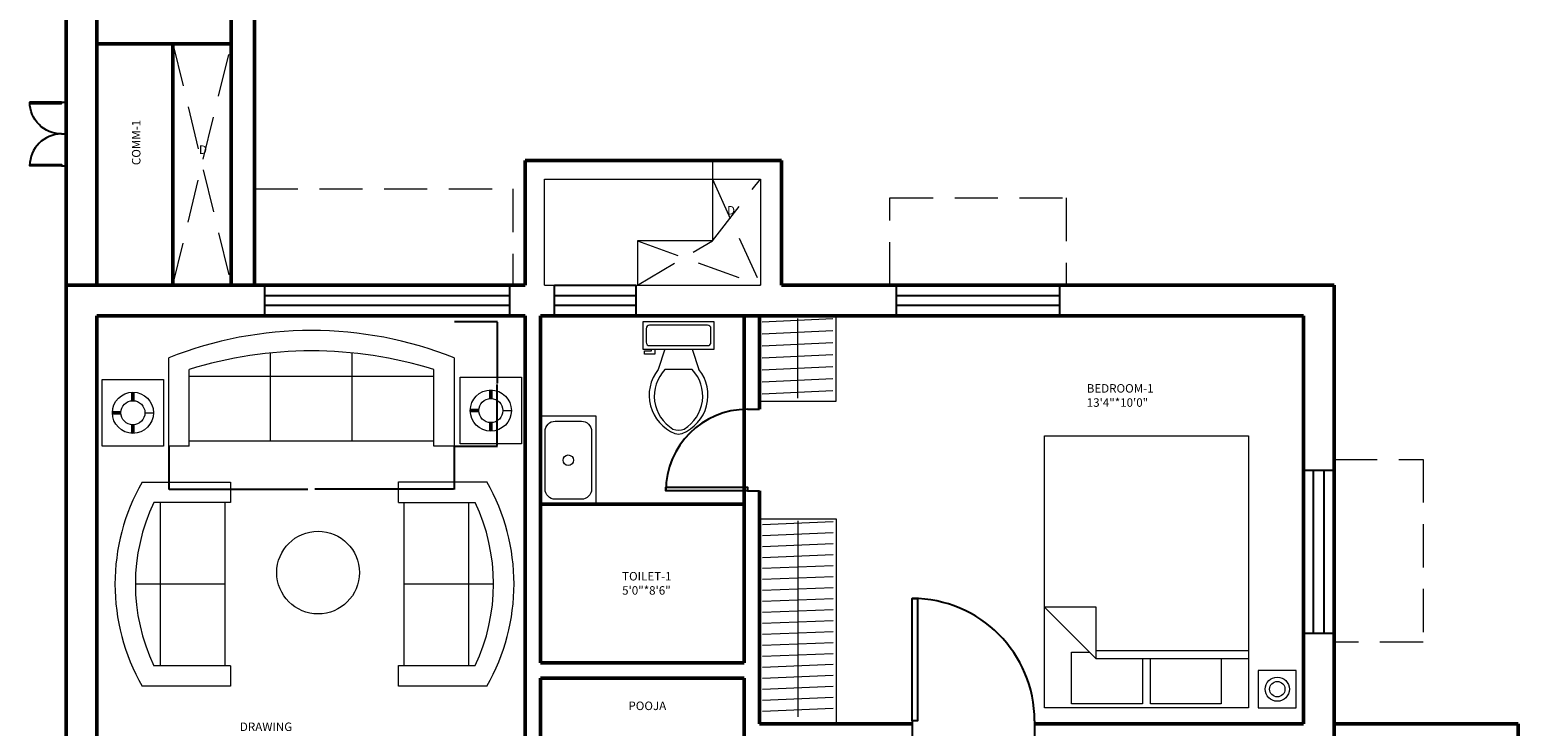
# Model space of a CAD drawing. Units: inches. Extents: x 4795 to 6024, y 2716 to 5025.
# Tile 8 of 19: x 5517 to 5955, y 3611 to 3816. Entities that reach past the tile are written whole.
import ezdxf

# ---------------------------------------------------------------- set-up
doc = ezdxf.new("R2010")
doc.units = ezdxf.units.IN
doc.linetypes.add('DASHED', pattern=[19.05, 12.7, -6.35])
for name, color, linetype, lineweight in [('A-ANNO-DIMS', 2, 'Continuous', 18), ('A-ANNO-TEXT', 7, 'Continuous', 18), ('A-AREA-IDEN', 3, 'Continuous', 18), ('A-DOOR', 4, 'Continuous', 25), ('A-FLOR-FIXT', 9, 'Continuous', 18), ('A-FURN', 8, 'Continuous', 18), ('A-GLAZ', 4, 'Continuous', 25), ('A-WALL', 7, 'Continuous', 50), ('A-WALL-OVHD', 8, 'DASHED', 18)]:
    doc.layers.add(name, color=color, linetype=linetype, lineweight=lineweight)
doc.styles.get("Standard").update_dxf_attribs({"font": 'arial.ttf'})
doc.dimstyles.get("Standard").update_dxf_attribs({"dimtxt": 0.18, "dimasz": 0.18, "dimexe": 0.18, "dimexo": 0.0625, "dimgap": 0.09, "dimtad": 0, "dimtih": 1, "dimtoh": 1, "dimdec": 4, "dimzin": 0, "dimdsep": 46, "dimtxsty": 'Standard', "dimcen": 0.09, "dimadec": 0, "dimazin": 0, "dimtfac": 1, "dimtdec": 4, "dimtofl": 0, "dimtmove": 0, "dimatfit": 3, "dimfxl": 1, "dimtolj": 1, "dimtzin": 0, "dimarcsym": 0})

# ---------------------------------------------------------------- blocks, each defined once
blk = doc.blocks.new('*U2')
for p, q in [((0, 0), (0, -6)), ((40, 0), (40, -6))]:
    blk.add_line(p, q)
blk.add_lwpolyline([(0, 0), (0, 40), (1.75, 40), (1.75, 0)], close=True)
blk.add_arc((0, 0), 40, 0, 90)
blk = doc.blocks.new('Sofa - Roundback 7 ft.')
for p, q in [((-12.00002, -32.4421), (-12.00003, -6.5971)), ((11.99997, -32.4421), (11.99998, -6.5971)), ((-36.000027, -34), (-36.000027, -11.4696)), ((35.99998, -34), (35.99998, -11.4696)), ((-35.999844, -13.3819), (35.9998, -13.3819)), ((-36.000027, -32.4421), (35.99998, -32.4421))]:
    blk.add_line(p, q)
for points in [[(-36.000027, -34), (-42.000027, -34), (-42.000027, -8)], [(41.99998, -8), (41.99998, -34), (35.99998, -34)]]:
    blk.add_lwpolyline(points)
for centre, radius, start, end in [((0, -114.25), 114.25, 68.43141, 111.5686), ((-0.00001, -127.1968), 121.1968, 72.72033, 107.2797)]:
    blk.add_arc(centre, radius, start, end)
blk = doc.blocks.new('Sofa - Roundback Loveseat 5 ft.')
for p, q in [((0, -32.44198), (0, -5.99998)), ((-24, -33.99998), (-24, -11.46958)), ((24.00004, -33.99998), (24.00004, -11.46958)), ((-23.9998, -13.38178), (23.99986, -13.38178)), ((-24, -32.44198), (24.00004, -32.44198))]:
    blk.add_line(p, q)
for points in [[(-24, -33.99998), (-30, -33.99998), (-30, -7.99998)], [(30.00004, -7.99998), (30.00004, -33.99998), (24.00004, -33.99998)]]:
    blk.add_lwpolyline(points)
for centre, radius, start, end in [((0, -60.24998), 60.24998, 60.13715, 119.8628), ((0, -61.38438), 55.38444, 64.32083, 115.6792)]:
    blk.add_arc(centre, radius, start, end)
blk = doc.blocks.new('Toilet - top')
for p, q in [((9.5, -6), (9.5, -2)), ((-10, -8.5), (-8, -8.5)), ((-10, -9.5), (-10, -8.5)), ((-8, -8.5), (-8, -8)), ((-7, -8), (-7, -9.5)), ((-4, -8), (-6, -14)), ((4, -8), (6, -14)), ((-7, -9.5), (-10, -9.5)), ((4, -14), (-4, -14))]:
    blk.add_line(p, q)
blk.add_lwpolyline([(10.5, -8), (10.5, 0), (-10.5, 0), (-10.5, -8)], close=True)
for points in [[(-9.5, -2), (-9.5, -6)], [(8.5, -1), (-8.5, -1)], [(-8.5, -7), (8.5, -7)]]:
    blk.add_lwpolyline(points)
for centre, radius, start, end in [((-8.62, -1.88), 0.884, 81.8699, 188.1301), ((8.62, -1.88), 0.884, 351.8699, 98.1301), ((-8.62, -6.12), 0.884, 171.8699, 278.1301), ((8.62, -6.12), 0.884, 261.8699, 8.1301), ((3.52, -21.58), 12.17, 141.4691, 247.9714), ((4.2, -21.82), 11.33, 136.3677, 238.9468), ((-3.52, -21.58), 12.17, 292.0284, 38.5307), ((-4.2, -21.82), 11.33, 301.053, 43.6321), ((0, -27.88), 4, 245.7318, 294.2682), ((0, -29), 4, 254.8605, 285.1395)]:
    blk.add_arc(centre, radius, start, end)
blk = doc.blocks.new('Bed - Queen')
for p, q in [((0, -80.00003), (0, 0)), ((0, 0), (59.99999, 0)), ((59.99999, 0), (59.99999, -80.00003)), ((7.99999, -1.2), (28.79998, -1.2)), ((7.99999, -14.4), (7.99999, -1.2)), ((28.79998, -1.2), (28.79998, -14.4)), ((31.19999, -1.2), (51.99999, -1.2)), ((31.19999, -14.4), (31.19999, -1.2)), ((51.99999, -1.2), (51.99999, -16.4)), ((0, -14.4), (44.8, -14.4)), ((44.8, -16.8), (0, -16.8)), ((59.99999, -29.6), (44.8, -14.4)), ((44.8, -14.4), (44.8, -29.6)), ((51.99999, -16.4), (46.79936, -16.4)), ((44.8, -29.6), (59.99999, -29.6)), ((59.99999, -80.00003), (0, -80.00003))]:
    blk.add_line(p, q)
blk = doc.blocks.new('WIN-48')
for p, q in [((0, 0), (0, 48)), ((0, 48), (9, 48)), ((3, 0), (3, 48)), ((6, 48), (6, 0)), ((9, 48), (9, 0)), ((9, 0), (0, 0))]:
    blk.add_line(p, q)
blk = doc.blocks.new('WIN-72')
for p, q in [((0, 0), (0, 9)), ((0, 9), (72, 9)), ((72, 9), (72, 0)), ((0, 6), (72, 6)), ((72, 3), (0, 3)), ((72, 0), (0, 0))]:
    blk.add_line(p, q)
blk = doc.blocks.new('WIN-24')
for p, q in [((0, 0), (0, 9)), ((0, 9), (24, 9)), ((24, 9), (24, 0)), ((0, 6), (24, 6)), ((24, 3), (0, 3)), ((24, 0), (0, 0))]:
    blk.add_line(p, q)
blk = doc.blocks.new('*D41')
at = {"layer": 'A-ANNO-DIMS', "color": 0, "lineweight": -2, "transparency": 16777216}
for p, q in [((5558.35, 3693.06), (5558.35, 3680.34)), ((5642.35, 3693.06), (5642.35, 3680.34)), ((5558.53, 3680.52), (5599.32, 3680.52)), ((5642.17, 3680.52), (5601.38, 3680.52))]:
    blk.add_line(p, q, dxfattribs=at)
at = {"layer": 'A-ANNO-DIMS', "color": 0, "lineweight": 100, "transparency": 16777216}
for points in [[(5558.53, 3680.55), (5558.53, 3680.49), (5558.35, 3680.52)], [(5642.17, 3680.55), (5642.17, 3680.49), (5642.35, 3680.52)]]:
    blk.add_solid(points, dxfattribs=at)
at = {"layer": 'DEFPOINTS', "color": 0, "lineweight": 100, "transparency": 16777216}
for p in [(5558.35, 3693.12), (5642.35, 3693.12), (5642.35, 3680.52)]:
    blk.add_point(p, dxfattribs=at)
at = {"layer": 'A-ANNO-DIMS', "color": 0, "transparency": 16777216, "insert": (5600.35, 3680.52), "char_height": 0.18, "attachment_point": 5}
blk.add_mtext("\\A1;SOFA 7' 84 TYP.", dxfattribs=at)
blk = doc.blocks.new('*D42')
at = {"layer": 'A-ANNO-DIMS', "color": 0, "lineweight": -2, "transparency": 16777216}
for p, q in [((5642.41, 3729.79), (5655.13, 3729.79)), ((5654.95, 3729.61), (5654.95, 3711.64)), ((5654.95, 3693.3), (5654.95, 3711.28)), ((5642.41, 3693.12), (5655.13, 3693.12))]:
    blk.add_line(p, q, dxfattribs=at)
at = {"layer": 'A-ANNO-DIMS', "color": 0, "lineweight": 100, "transparency": 16777216}
for points in [[(5654.92, 3729.61), (5654.98, 3729.61), (5654.95, 3729.79)], [(5654.92, 3693.3), (5654.98, 3693.3), (5654.95, 3693.12)]]:
    blk.add_solid(points, dxfattribs=at)
at = {"layer": 'DEFPOINTS', "color": 0, "lineweight": 100, "transparency": 16777216}
for p in [(5642.35, 3729.79), (5654.95, 3729.79), (5642.35, 3693.12)]:
    blk.add_point(p, dxfattribs=at)
at = {"layer": 'A-ANNO-DIMS', "color": 0, "transparency": 16777216, "insert": (5654.95, 3711.46), "char_height": 0.18, "attachment_point": 5}
blk.add_mtext('\\A1;37 TYP.', dxfattribs=at)

msp = doc.modelspace()

# ---------------------------------------------------------------- linework, layer by layer
at = {"layer": 'A-FLOR-FIXT'}
msp.add_lwpolyline([(5667.72, 3676.04), (5684.08, 3676.04), (5684.08, 3701.96), (5667.72, 3701.96)], close=True, dxfattribs=at)
msp.add_lwpolyline([(5672.08, 3700.46), (5679.77, 3700.46, -0.414214), (5682.77, 3697.46), (5682.77, 3680.5, -0.414214), (5679.77, 3677.5), (5672.08, 3677.5, -0.414214), (5669.08, 3680.5), (5669.08, 3697.46, -0.414214)], format="xyb", close=True, dxfattribs=at)
msp.add_circle((5675.92, 3688.98), 1.55, dxfattribs=at)
at = {"layer": 'A-FURN'}
for p, q in [((5718.34, 3777.12), (5718.34, 3771.66)), ((5668.93, 3740.43), (5668.93, 3771.66)), ((5668.93, 3771.66), (5732.5, 3771.66)), ((5718.34, 3771.66), (5718.34, 3753.53)), ((5732.5, 3771.66), (5732.5, 3740.43)), ((5718.34, 3753.53), (5696.25, 3753.53)), ((5696.25, 3753.53), (5696.25, 3740.43)), ((5668.93, 3740.43), (5732.5, 3740.43)), ((5754.73, 3706.3), (5754.73, 3731.43)), ((5732.94, 3729.68), (5753.73, 3730.61)), ((5732.94, 3726.15), (5753.73, 3727.08)), ((5743.33, 3730.69), (5743.33, 3707.22)), ((5732.94, 3722.62), (5753.73, 3723.55)), ((5732.94, 3719.1), (5753.73, 3720.03)), ((5732.94, 3715.57), (5753.73, 3716.5)), ((5732.94, 3712.05), (5753.73, 3712.98)), ((5732.22, 3706.3), (5754.73, 3706.3)), ((5732.94, 3708.52), (5753.73, 3709.45)), ((5551.36, 3702.94), (5553.87, 3702.94)), ((5656.67, 3703.58), (5659.18, 3703.58)), ((5732.22, 3671.71), (5754.73, 3671.71)), ((5733.04, 3670.11), (5753.82, 3670.93)), ((5743.43, 3671.14), (5743.43, 3613.55)), ((5754.73, 3671.71), (5754.73, 3611.43)), ((5733.04, 3666.88), (5753.82, 3667.7)), ((5733.04, 3663.66), (5753.82, 3664.48)), ((5733.04, 3660.43), (5753.82, 3661.25)), ((5733.04, 3657.2), (5753.82, 3658.02)), ((5733.04, 3653.97), (5753.82, 3654.79)), ((5733.04, 3650.74), (5753.82, 3651.56)), ((5733.04, 3647.52), (5753.82, 3648.34)), ((5733.04, 3644.29), (5753.82, 3645.11)), ((5733.04, 3641.06), (5753.82, 3641.88)), ((5733.04, 3637.83), (5753.82, 3638.65)), ((5733.04, 3634.6), (5753.82, 3635.42)), ((5733.04, 3631.38), (5753.82, 3632.2)), ((5733.04, 3628.15), (5753.82, 3628.97)), ((5733.04, 3624.92), (5753.82, 3625.74)), ((5733.04, 3621.69), (5753.82, 3622.51)), ((5733.04, 3618.46), (5753.82, 3619.28)), ((5733.04, 3615.24), (5753.82, 3616.06))]:
    msp.add_line(p, q, dxfattribs=at)
for points in [[(5556.84, 3693.12), (5538.81, 3693.12), (5538.81, 3712.75), (5556.84, 3712.75)], [(5662.14, 3693.77), (5644.11, 3693.77), (5644.11, 3713.4), (5662.14, 3713.4)], [(5878.95, 3616.19), (5890.13, 3616.19), (5890.13, 3627.14), (5878.95, 3627.14)]]:
    msp.add_lwpolyline(points, close=True, dxfattribs=at)
for centre, radius in [((5653.13, 3703.58), 6.05), ((5547.82, 3702.94), 6.05), ((5547.82, 3702.94), 3.54), ((5653.13, 3703.58), 3.54), ((5602.31, 3655.94), 12.16), ((5884.54, 3621.66), 3.55), ((5884.54, 3621.66), 2.26)]:
    msp.add_circle(centre, radius, dxfattribs=at)
at = {"layer": 'A-WALL'}
for p, q in [((5537.22, 3929.81), (5537.22, 3740.43)), ((5528.22, 3920.81), (5528.22, 3351.93)), ((5576.74, 3920.81), (5576.74, 3740.43)), ((5583.63, 3920.81), (5583.63, 3740.43)), ((5537.22, 3811.38), (5576.74, 3811.38)), ((5559.58, 3811.38), (5559.58, 3740.43)), ((5663.22, 3740.43), (5663.22, 3777.12)), ((5663.22, 3777.12), (5732.22, 3777.12)), ((5732.22, 3777.12), (5738.7, 3777.12)), ((5738.7, 3777.12), (5738.7, 3740.43)), ((5528.22, 3740.43), (5663.22, 3740.43)), ((5738.7, 3740.43), (5901.22, 3740.43)), ((5901.22, 3740.43), (5901.22, 3606.93)), ((5537.22, 3731.43), (5663.22, 3731.43)), ((5537.22, 3731.43), (5537.22, 3551.43)), ((5663.22, 3731.43), (5663.22, 3606.93)), ((5667.72, 3731.43), (5667.72, 3629.43)), ((5667.72, 3731.43), (5892.22, 3731.43)), ((5727.72, 3731.43), (5727.72, 3629.43)), ((5732.22, 3731.43), (5732.22, 3703.97)), ((5892.22, 3731.43), (5892.22, 3611.43)), ((5653.13, 3709.64), (5653.13, 3707.12)), ((5547.82, 3708.99), (5547.82, 3706.48)), ((5541.77, 3702.94), (5544.28, 3702.94)), ((5647.07, 3703.58), (5649.59, 3703.58)), ((5547.82, 3699.4), (5547.82, 3696.88)), ((5653.13, 3700.04), (5653.13, 3697.53)), ((5732.22, 3679.97), (5732.22, 3611.43)), ((5667.72, 3676.04), (5727.72, 3676.04)), ((5667.72, 3629.43), (5727.72, 3629.43)), ((5667.72, 3624.93), (5727.72, 3624.93)), ((5667.72, 3624.93), (5667.72, 3606.93)), ((5727.72, 3624.93), (5727.72, 3606.93)), ((5732.22, 3611.43), (5777.13, 3611.43)), ((5813.13, 3611.43), (5892.22, 3611.43)), ((5901.22, 3611.43), (5955.43, 3611.43)), ((5955.43, 3611.43), (5955.43, 3483.93))]:
    msp.add_line(p, q, dxfattribs=at)
at = {"layer": 'A-WALL-OVHD'}
for p, q in [((5559.58, 3811.38), (5576.74, 3740.43)), ((5559.58, 3740.43), (5576.74, 3811.38)), ((5718.34, 3771.66), (5732.5, 3740.43)), ((5718.34, 3753.53), (5732.5, 3771.66)), ((5583.63, 3768.75), (5659.62, 3768.75)), ((5659.62, 3768.75), (5659.62, 3740.43)), ((5770.58, 3740.43), (5770.58, 3766.11)), ((5770.58, 3766.11), (5822.43, 3766.11)), ((5822.43, 3766.11), (5822.43, 3740.43)), ((5696.25, 3753.53), (5732.5, 3740.43)), ((5696.25, 3740.43), (5718.34, 3753.53)), ((5901.22, 3689.24), (5927.44, 3689.24)), ((5927.44, 3689.24), (5927.44, 3635.48)), ((5927.44, 3635.48), (5901.22, 3635.48))]:
    msp.add_line(p, q, dxfattribs=at)

# ---------------------------------------------------------------- block references
at = {"layer": 'A-DOOR'}
for p, xscale, yscale, zscale, rotation in [((5526.82, 3794.26), -0.2337145210718518, 0.2337145210718518, 0.2337145210718518, 90), ((5526.82, 3775.56), 0.2337145210718518, 0.2337145210718518, 0.2337145210718518, 89.99999999999999), ((5728.62, 3679.97), 0.6, 0.6, 0.6, 90.00000000000003)]:
    msp.add_blockref('*U2', p, dxfattribs=dict(at, xscale=xscale, yscale=yscale, zscale=zscale, rotation=rotation))
at = {"layer": 'A-DOOR', "xscale": 0.9, "yscale": 0.9, "zscale": 0.9}
msp.add_blockref('*U2', (5777.13, 3612.33), dxfattribs=at)
at = {"layer": 'A-FLOR-FIXT'}
msp.add_blockref('Toilet - top', (5708.36, 3729.67), dxfattribs=at)
at = {"layer": 'A-FURN'}
msp.add_blockref('Sofa - Roundback 7 ft.', (5600.35, 3727.12), dxfattribs=at)
for name, p, rotation in [('Bed - Queen', (5876.03, 3616.19), 180), ('Sofa - Roundback Loveseat 5 ft.', (5542.54, 3652.57), 90), ('Sofa - Roundback Loveseat 5 ft.', (5659.95, 3652.59), 270)]:
    msp.add_blockref(name, p, dxfattribs=dict(at, rotation=rotation))
at = {"layer": 'A-GLAZ'}
for name, p, rotation in [('WIN-72', (5658.67, 3740.43), 180), ('WIN-24', (5695.82, 3740.43), 180), ('WIN-48', (5820.49, 3731.43), 90.00000000000036)]:
    msp.add_blockref(name, p, dxfattribs=dict(at, rotation=rotation))
msp.add_blockref('WIN-48', (5892.22, 3638.07), dxfattribs=at)

# ---------------------------------------------------------------- texts
at = {"layer": 'A-ANNO-TEXT', "insert": (5547.54, 3775.75), "char_height": 2.5, "attachment_point": 1, "rotation": 90}
msp.add_mtext_dynamic_manual_height_columns('COMM-1', width=16.0113, gutter_width=12.5, heights=[0], dxfattribs=at)
at = {"layer": 'A-ANNO-TEXT', "char_height": 2.5, "attachment_point": 1}
for width, insert in [(1.3185, (5567.25, 3781.54)), (2.275, (5722.64, 3763.73))]:
    msp.add_mtext_dynamic_manual_height_columns('D', width=width, gutter_width=12.5, heights=[0], dxfattribs=dict(at, insert=insert))
at = {"layer": 'A-AREA-IDEN', "char_height": 2.5, "attachment_point": 1}
for s, width, insert in [('BEDROOM-1\\P13\'4"*10\'0"', 68.948, (5828.47, 3711.36)), ('TOILET-1\\P5\'0"*8\'6"', 47.9474, (5691.76, 3656.12)), ('POOJA', 33.5958, (5693.62, 3618.02)), ('DRAWING\\P10\'6"*15\'0"', 61.2488, (5579.3, 3611.86))]:
    msp.add_mtext_dynamic_manual_height_columns(s, width=width, gutter_width=12.5, heights=[0], dxfattribs=dict(at, insert=insert))

# ---------------------------------------------------------------- dimensions: what is measured, and where the dimension line sits
at = {"layer": 'A-ANNO-DIMS'}
dim = msp.add_linear_dim(base=(5654.95, 3729.79), p1=(5642.35, 3693.12), p2=(5642.35, 3729.79), angle=90, text='<> TYP.', dimstyle='Standard', override={"dimdec": 0, "dimlfac": 1, "dimrnd": 0, "dimzin": 0, "dimdsep": 46, "dimlunit": 2}, dxfattribs=at)
dim.commit()
dim.dimension.update_dxf_attribs({"geometry": '*D42', "text_midpoint": (5654.95, 3711.46)})
dim = msp.add_linear_dim(base=(5642.35, 3680.52), p1=(5558.35, 3693.12), p2=(5642.35, 3693.12), text="SOFA 7' <> TYP.", dimstyle='Standard', override={"dimdec": 0, "dimlfac": 1, "dimrnd": 0, "dimzin": 0, "dimdsep": 46, "dimlunit": 2}, dxfattribs=at)
dim.commit()
dim.dimension.update_dxf_attribs({"geometry": '*D41', "text_midpoint": (5600.35, 3680.52)})

doc.saveas('drawing.dxf')
